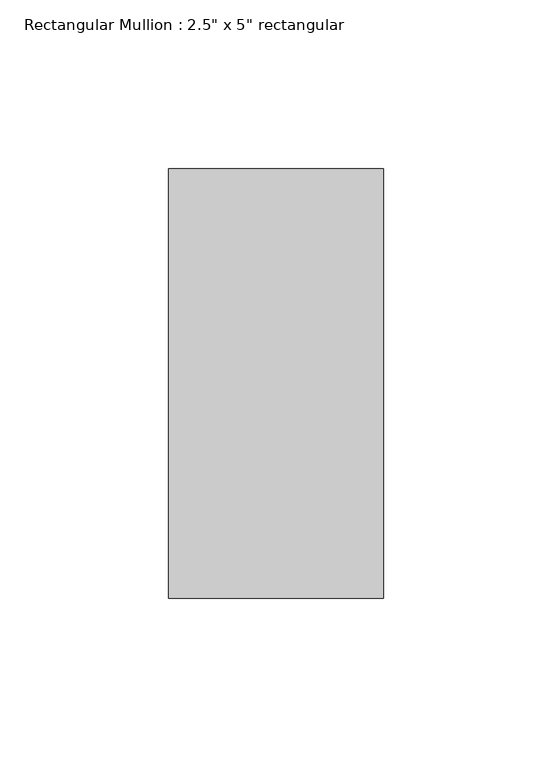
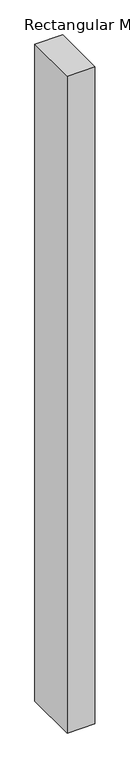
"""IFC4 building model written with IfcOpenShell, lengths in millimetres: member geometry."""

from ifc_helpers import new_model, si_unit, frame, origin, place, context, project, spatial, polyline, outline, extrude, source, transform, mapped, element, save


def member_082242e3(model_context):
    return source(origin(), model_context, "Body", "SweptSolid", [
        extrude(outline(polyline([(31.75, 63.5), (31.75, -63.5), (-31.75, -63.5), (-31.75, 63.5), (31.75, 63.5)])), frame((0.0, 0.0, -1586.1267095), z_axis=(0.0, 0.0, 1.0), x_axis=(1.0, 0.0, 0.0)), (0.0, 0.0, 1.0), 1586.1267095),
    ])


if __name__ == "__main__":
    model = new_model("IFC4")
    model_context = context("Model", 3, world=origin())
    ifc_project = project(units=[si_unit("LENGTHUNIT", "METRE", prefix="MILLI")], contexts=[model_context])
    site = spatial("IfcSite", under=ifc_project)
    building = spatial("IfcBuilding", under=site)
    placement = place(None, origin())
    member_shape = member_082242e3(model_context)
    element("IfcMember", 1, ObjectType="Rectangular Mullion : 2.5\" x 5\" rectangular", at=placement, inside=building, context=model_context, shape_type="MappedRepresentation", body=[
        mapped(member_shape, transform((0.0, 0.0, 0.0), x_axis=(1.0, 0.0, 0.0), y_axis=(0.0, 1.0, 0.0), z_axis=(0.0, 0.0, 1.0))),
    ])
    save(model, "model.ifc")

# Revit data of these elements
# Type "Rectangular Mullion : 2.5\" x 5\" rectangular"
#   built-in parameter 1007304 = 0.416667 (stored number, unit not read)
#   built-in parameter 1007301 = 0.104167 (stored number, unit not read)
#   built-in parameter 1007300 = 0.104167 (stored number, unit not read)
# Element 1 (IfcMember, "Rectangular Mullion : 2.5\" x 5\" rectangular")
#   Materials on its faces: "Aluminum"
# Materials
#   "Aluminum": class "Metal", colour RGB 247 247 247, transparency 0, Description = "Aluminum 6061", Cost = 0
